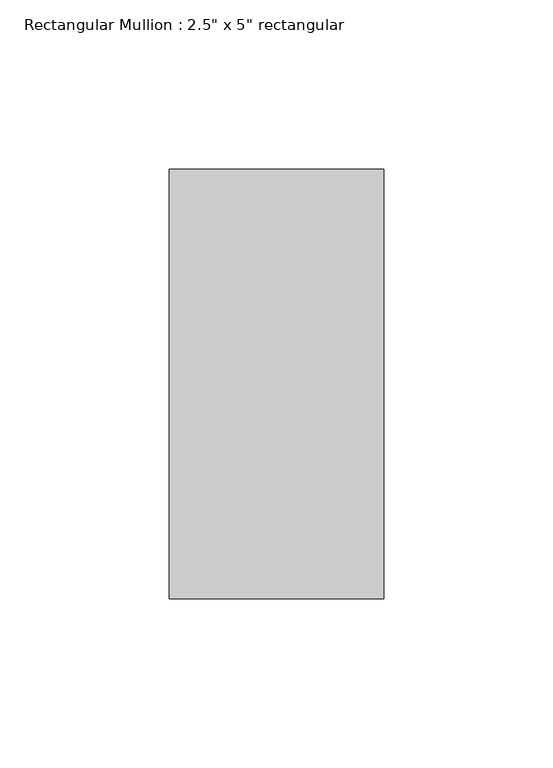
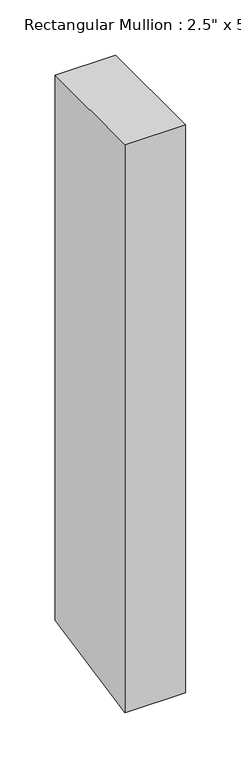
"""IFC4 building model written with IfcOpenShell, lengths in millimetres: member geometry."""

from ifc_helpers import new_model, si_unit, frame, origin, place, context, project, spatial, polyline, outline, extrude, source, transform, mapped, element, save


def member_e6e8f276(model_context):
    return source(origin(), model_context, "Body", "SweptSolid", [
        extrude(outline(polyline([(-63.5, 0.0), (63.5, 0.0), (63.5, -602.7536382), (-63.5, -628.0155089), (-63.5, 0.0)])), frame((-63.5, 0.0, 0.0), z_axis=(1.0, 0.0, 0.0), x_axis=(0.0, 1.0, 0.0)), (0.0, 0.0, 1.0), 63.5),
    ])


if __name__ == "__main__":
    model = new_model("IFC4")
    model_context = context("Model", 3, world=origin())
    ifc_project = project(units=[si_unit("LENGTHUNIT", "METRE", prefix="MILLI")], contexts=[model_context])
    site = spatial("IfcSite", under=ifc_project)
    building = spatial("IfcBuilding", under=site)
    placement = place(None, origin())
    member_shape = member_e6e8f276(model_context)
    element("IfcMember", 1, ObjectType="Rectangular Mullion : 2.5\" x 5\" rectangular", at=placement, inside=building, context=model_context, shape_type="MappedRepresentation", body=[
        mapped(member_shape, transform((0.0, 0.0, 0.0), x_axis=(1.0, 0.0, 0.0), y_axis=(0.0, 1.0, 0.0), z_axis=(0.0, 0.0, 1.0))),
    ])
    save(model, "model.ifc")

# Revit data of these elements
# Type "Rectangular Mullion : 2.5\" x 5\" rectangular"
#   built-in parameter 1007304 = 0.416667 (stored number, unit not read)
#   built-in parameter 1007301 = 0.104167 (stored number, unit not read)
#   built-in parameter 1007300 = 0.104167 (stored number, unit not read)
# Element 1 (IfcMember, "Rectangular Mullion : 2.5\" x 5\" rectangular")
#   Materials on its faces: "Iron, Ductile"
# Materials
#   "Iron, Ductile": class "Metal", colour RGB 0 0 0, transparency 0, Description = "Ductile cast iron", Cost = 0
